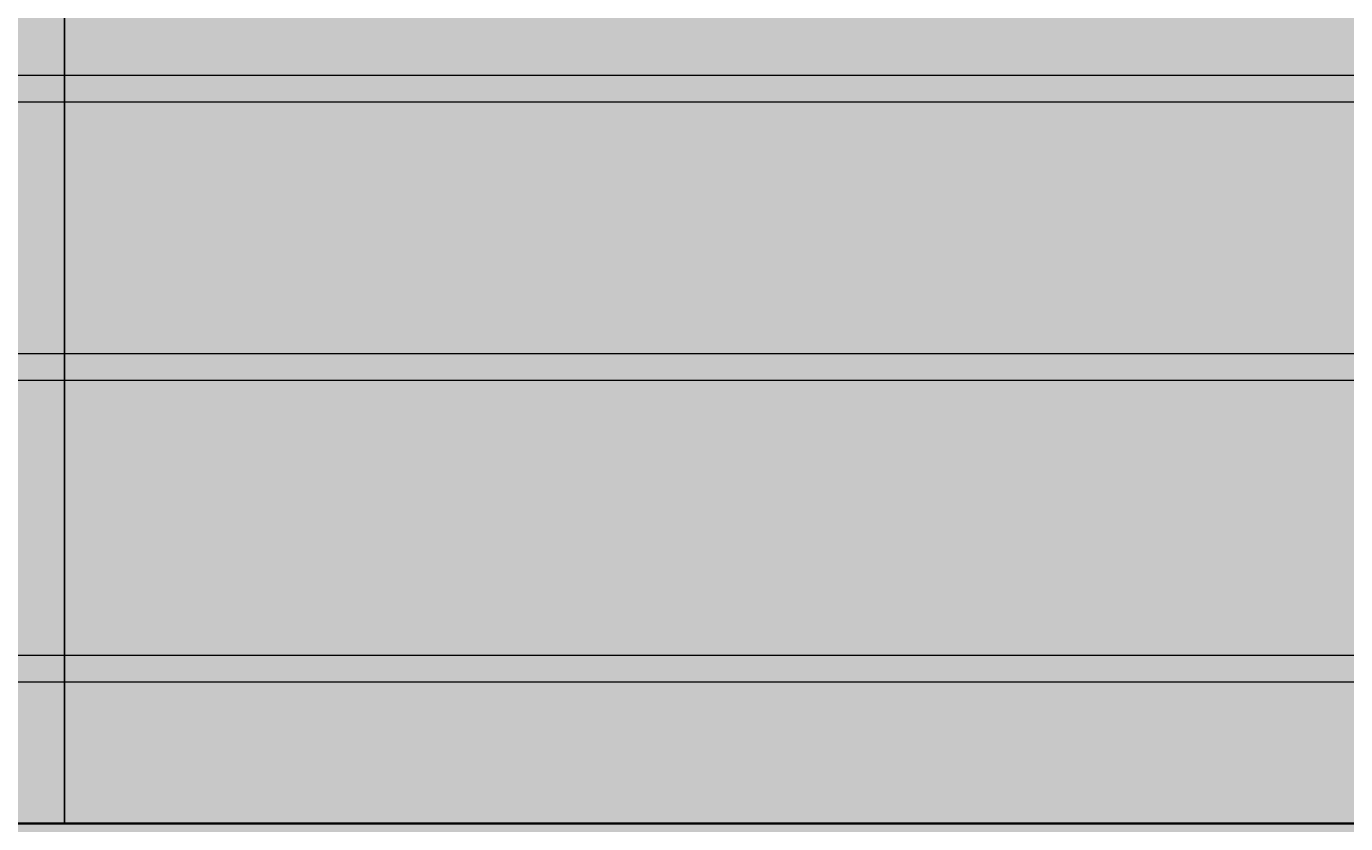
# Model space of a CAD drawing. Units: feet. Extents: x 2695 to 2912, y 795 to 1139.
# Tile 57 of 83: x 2843 to 2877, y 937 to 958. Entities that reach past the tile are written whole.
import ezdxf

# ---------------------------------------------------------------- set-up
doc = ezdxf.new("R2010")
doc.units = ezdxf.units.FT
for name, color, linetype, lineweight in [('A-ANNO-DIMS', 2, 'Continuous', 18), ('A-ELEV', 7, 'Continuous', 35), ('A-ELEV-PATT', 252, 'Continuous', 13), ('A-ELEV-RAIL', 8, 'Continuous', 18), ('A-GLAZ', 4, 'Continuous', 25)]:
    doc.layers.add(name, color=color, linetype=linetype, lineweight=lineweight)
doc.styles.get("Standard").update_dxf_attribs({"font": 'arial.ttf'})
doc.dimstyles.get("Standard").update_dxf_attribs({"dimtxt": 0.18, "dimasz": 0.18, "dimexe": 0.18, "dimexo": 0.0625, "dimgap": 0.09, "dimtad": 0, "dimtih": 1, "dimtoh": 1, "dimdec": 1, "dimzin": 0, "dimdsep": 46, "dimlunit": 3, "dimtxsty": 'Standard', "dimcen": 0.09, "dimadec": 0, "dimazin": 0, "dimtfac": 1, "dimtdec": 1, "dimtofl": 0, "dimtmove": 0, "dimatfit": 3, "dimfxl": 1, "dimtolj": 1, "dimtzin": 0, "dimarcsym": 0})

# ---------------------------------------------------------------- blocks, each defined once
blk = doc.blocks.new('*D17')
at = {"layer": 'A-ANNO-DIMS', "color": 0, "lineweight": -2, "transparency": 16777216}
for p, q in [((2843.637, 1020.824), (2911.424, 1020.824)), ((2911.244, 1020.644), (2911.244, 979.059)), ((2911.244, 937.111), (2911.244, 978.695)), ((2890.699, 936.931), (2911.424, 936.931))]:
    blk.add_line(p, q, dxfattribs=at)
at = {"layer": 'A-ANNO-DIMS', "color": 0, "transparency": 16777216}
for points in [[(2911.214, 1020.644), (2911.274, 1020.644), (2911.244, 1020.824)], [(2911.214, 937.111), (2911.274, 937.111), (2911.244, 936.931)]]:
    blk.add_solid(points, dxfattribs=at)
at = {"layer": 'Defpoints', "color": 0, "transparency": 16777216}
for p in [(2843.575, 1020.824), (2911.244, 1020.824), (2890.636, 936.931)]:
    blk.add_point(p, dxfattribs=at)
at = {"layer": 'A-ANNO-DIMS', "color": 0, "transparency": 16777216, "insert": (2911.244, 978.877), "char_height": 0.18, "attachment_point": 5}
blk.add_mtext('\\A1;83.9', dxfattribs=at)

msp = doc.modelspace()

# ---------------------------------------------------------------- hatches: boundary and pattern name
at = {"layer": 'A-ELEV-PATT'}
h = msp.add_hatch(color=256, dxfattribs=at)
h.set_gradient(color1=(255, 255, 255), tint=1)
h.paths.add_polyline_path([(2770.6361, 1122.9306), (2710.6361, 1122.9306), (2710.6361, 1118.4096), (2770.6361, 1118.4096)])
h.paths.add_polyline_path([(2890.6361, 1107.8588), (2770.6361, 1107.8588), (2770.6361, 1103.3378), (2890.6361, 1103.3378)])
h.paths.add_polyline_path([(2890.6361, 1062.9306), (2710.6361, 1062.9306), (2710.6361, 1056.9306), (2710.6361, 936.9306), (2710.6361, 924.3105), (2716.5358, 924.3105), (2890.6361, 924.3105), (2890.6361, 936.9306), (2715.8852, 936.9306), (2715.8852, 1050.3105), (2890.6361, 1050.3105)])
h.paths.add_polyline_path([(2716.5358, 924.3105), (2710.6361, 924.3105), (2710.6361, 810.9306), (2716.5358, 810.9306)])
h = msp.add_hatch(color=256, dxfattribs=at)
h.set_gradient(color1=(147, 149, 152), color2=(147, 149, 152), tint=1)
h.paths.add_polyline_path([(2770.6361, 1118.4096), (2710.6361, 1118.4096), (2710.6361, 1062.9306), (2770.6361, 1062.9306)])
h.paths.add_polyline_path([(2890.6361, 1103.3378), (2770.6361, 1103.3378), (2770.6361, 1062.9306), (2890.6361, 1062.9306)])
h.paths.add_polyline_path([(2730.7081, 1048.1052), (2755.1125, 1048.1052), (2755.1125, 936.9306), (2770.6361, 936.9306), (2770.6361, 1050.3105), (2715.8852, 1050.3105), (2715.8852, 936.9306), (2730.7081, 936.9306)])
h.paths.add_polyline_path([(2890.6361, 1050.3105), (2770.6361, 1050.3105), (2770.6361, 971.9673), (2778.0341, 971.9673), (2778.0341, 1020.8235), (2843.575, 1020.8235), (2843.575, 971.9673), (2890.6361, 971.9673)])
h.paths.add_polyline_path([(2888.1882, 970.7156), (2843.575, 970.7156), (2843.575, 964.8267), (2888.1882, 964.8267)])
h.paths.add_polyline_path([(2888.1882, 964.1328), (2843.575, 964.1328), (2843.575, 956.614), (2888.1882, 956.614)])
h.paths.add_polyline_path([(2888.1882, 955.9202), (2843.575, 955.9202), (2843.575, 949.2892), (2888.1882, 949.2892)])
h.paths.add_polyline_path([(2888.1882, 948.5954), (2843.575, 948.5954), (2843.575, 941.3507), (2888.1882, 941.3507)])
h.paths.add_polyline_path([(2888.1882, 940.6569), (2843.575, 940.6569), (2843.575, 936.9306), (2888.1882, 936.9306)])
h.paths.add_polyline_path([(2890.6361, 970.7156), (2888.9368, 970.7156), (2888.9368, 964.8267), (2890.6361, 964.8267)])
h.paths.add_polyline_path([(2890.6361, 964.1328), (2888.9368, 964.1328), (2888.9368, 956.614), (2890.6361, 956.614)])
h.paths.add_polyline_path([(2890.6361, 955.9202), (2888.9368, 955.9202), (2888.9368, 949.2892), (2890.6361, 949.2892)])
h.paths.add_polyline_path([(2890.6361, 940.6569), (2888.9368, 940.6569), (2888.9368, 936.9306), (2890.6361, 936.9306)])
h.paths.add_polyline_path([(2890.6361, 948.5954), (2888.9368, 948.5954), (2888.9368, 941.3507), (2890.6361, 941.3507)])
h.paths.add_polyline_path([(2772.5216, 970.7156), (2770.6361, 970.7156), (2770.6361, 964.8267), (2772.5216, 964.8267)])
h.paths.add_polyline_path([(2772.5216, 964.1328), (2770.6361, 964.1328), (2770.6361, 956.614), (2772.5216, 956.614)])
h.paths.add_polyline_path([(2772.5216, 955.9202), (2770.6361, 955.9202), (2770.6361, 949.2892), (2772.5216, 949.2892)])
h.paths.add_polyline_path([(2772.5216, 948.5954), (2770.6361, 948.5954), (2770.6361, 941.3507), (2772.5216, 941.3507)])
h.paths.add_polyline_path([(2772.5216, 940.6569), (2770.6361, 940.6569), (2770.6361, 936.9306), (2772.5216, 936.9306)])
h.paths.add_polyline_path([(2778.0341, 940.6569), (2773.2702, 940.6569), (2773.2702, 936.9306), (2778.0341, 936.9306)])
h.paths.add_polyline_path([(2778.0341, 970.7156), (2773.2702, 970.7156), (2773.2702, 964.8267), (2778.0341, 964.8267)])
h.paths.add_polyline_path([(2778.0341, 964.1328), (2773.2702, 964.1328), (2773.2702, 956.614), (2778.0341, 956.614)])
h.paths.add_polyline_path([(2778.0341, 955.9202), (2773.2702, 955.9202), (2773.2702, 949.2892), (2778.0341, 949.2892)])
h.paths.add_polyline_path([(2778.0341, 948.5954), (2773.2702, 948.5954), (2773.2702, 941.3507), (2778.0341, 941.3507)])
h.paths.add_polyline_path([(2810.0407, 940.6569), (2780.0341, 940.6569), (2780.0341, 936.9306), (2810.0407, 936.9306)])
h.paths.add_polyline_path([(2890.6361, 924.3105), (2770.6361, 924.3105), (2770.6361, 810.9306), (2773.5029, 810.9306), (2773.5029, 905.5143), (2805.9398, 905.5143), (2838.3767, 905.5143), (2838.3767, 810.9306), (2890.6361, 810.9306)])
h = msp.add_hatch(color=256, dxfattribs=at)
h.set_gradient(color2=(0, 0, 0), tint=1)
h.paths.add_polyline_path([(2772.5216, 971.9673), (2770.6361, 971.9673), (2770.6361, 970.7156), (2772.5216, 970.7156)])
h.paths.add_polyline_path([(2773.2702, 971.9673), (2772.5216, 971.9673), (2772.5216, 970.7156), (2773.2702, 970.7156)])
h.paths.add_polyline_path([(2778.0341, 971.9673), (2773.2702, 971.9673), (2773.2702, 970.7156), (2778.0341, 970.7156)])
h.paths.add_polyline_path([(2780.0341, 971.9673), (2778.0341, 971.9673), (2778.0341, 970.7156), (2780.0341, 970.7156)])
h.paths.add_polyline_path([(2841.575, 971.9673), (2780.0341, 971.9673), (2780.0341, 970.7156), (2841.575, 970.7156)])
h.paths.add_polyline_path([(2843.575, 971.9673), (2841.575, 971.9673), (2841.575, 970.7156), (2843.575, 970.7156)])
h.paths.add_polyline_path([(2888.1882, 971.9673), (2843.575, 971.9673), (2843.575, 970.7156), (2888.1882, 970.7156)])
h.paths.add_polyline_path([(2888.9368, 971.9673), (2888.1882, 971.9673), (2888.1882, 970.7156), (2888.9368, 970.7156)], flags=17)
h.paths.add_polyline_path([(2890.6361, 971.9673), (2888.9368, 971.9673), (2888.9368, 970.7156), (2890.6361, 970.7156)])
h.paths.add_polyline_path([(2888.9368, 971.9673), (2888.1882, 971.9673), (2888.1882, 964.8267), (2888.9368, 964.8267)])
h.paths.add_polyline_path([(2888.9368, 964.8267), (2888.1882, 964.8267), (2888.1882, 964.1328), (2888.9368, 964.1328)])
h.paths.add_polyline_path([(2890.6361, 964.8267), (2888.9368, 964.8267), (2888.9368, 964.1328), (2890.6361, 964.1328)])
h.paths.add_polyline_path([(2888.1882, 964.8267), (2770.6361, 964.8267), (2770.6361, 964.1328), (2888.1882, 964.1328)])
h.paths.add_polyline_path([(2888.9368, 964.1328), (2888.1882, 964.1328), (2888.1882, 936.9306), (2888.9368, 936.9306)])
h.paths.add_polyline_path([(2890.6361, 956.614), (2888.9368, 956.614), (2888.9368, 955.9202), (2890.6361, 955.9202)])
h.paths.add_polyline_path([(2888.1882, 956.614), (2770.6361, 956.614), (2770.6361, 955.9202), (2888.1882, 955.9202)])
h.paths.add_polyline_path([(2890.6361, 949.2892), (2888.9368, 949.2892), (2888.9368, 948.5954), (2890.6361, 948.5954)])
h.paths.add_polyline_path([(2888.1882, 949.2892), (2770.6361, 949.2892), (2770.6361, 948.5954), (2888.1882, 948.5954)])
h.paths.add_polyline_path([(2890.6361, 941.3507), (2888.9368, 941.3507), (2888.9368, 940.6569), (2890.6361, 940.6569)])
h.paths.add_polyline_path([(2888.1882, 941.3507), (2770.6361, 941.3507), (2770.6361, 940.6569), (2888.1882, 940.6569)])
h.paths.add_polyline_path([(2773.2702, 970.7156), (2772.5216, 970.7156), (2772.5216, 964.8267), (2773.2702, 964.8267)])
h.paths.add_polyline_path([(2773.2702, 964.1328), (2772.5216, 964.1328), (2772.5216, 956.614), (2773.2702, 956.614)])
h.paths.add_polyline_path([(2773.2702, 955.9202), (2772.5216, 955.9202), (2772.5216, 936.9306), (2773.2702, 936.9306)])
h.paths.add_polyline_path([(2810.7893, 970.7156), (2810.0407, 970.7156), (2810.0407, 964.8267), (2810.7893, 964.8267)], flags=17)
h.paths.add_polyline_path([(2810.7893, 964.1328), (2810.0407, 964.1328), (2810.0407, 956.614), (2810.7893, 956.614)], flags=17)
h.paths.add_polyline_path([(2810.7893, 955.9202), (2810.0407, 955.9202), (2810.0407, 949.2892), (2810.7893, 949.2892)], flags=17)
h.paths.add_polyline_path([(2810.7893, 971.9673), (2810.0407, 971.9673), (2810.0407, 941.3507), (2810.7893, 941.3507)])
h.paths.add_polyline_path([(2810.7893, 940.6569), (2810.0407, 940.6569), (2810.0407, 936.9306), (2810.7893, 936.9306)])
h.paths.add_polyline_path([(2780.0341, 1018.8235), (2841.575, 1018.8235), (2841.575, 971.9673), (2843.575, 971.9673), (2843.575, 1020.8235), (2778.0341, 1020.8235), (2778.0341, 971.9673), (2780.0341, 971.9673)])
h.paths.add_polyline_path([(2780.0341, 970.7156), (2778.0341, 970.7156), (2778.0341, 964.8267), (2780.0341, 964.8267)])
h.paths.add_polyline_path([(2780.0341, 964.1328), (2778.0341, 964.1328), (2778.0341, 956.614), (2780.0341, 956.614)])
h.paths.add_polyline_path([(2780.0341, 955.9202), (2778.0341, 955.9202), (2778.0341, 949.2892), (2780.0341, 949.2892)])
h.paths.add_polyline_path([(2780.0341, 948.5954), (2778.0341, 948.5954), (2778.0341, 941.3507), (2780.0341, 941.3507)])
h.paths.add_polyline_path([(2780.0341, 940.6569), (2778.0341, 940.6569), (2778.0341, 936.9306), (2780.0341, 936.9306)])
h.paths.add_polyline_path([(2843.575, 940.6569), (2841.575, 940.6569), (2841.575, 936.9306), (2843.575, 936.9306)])
h.paths.add_polyline_path([(2843.575, 948.5954), (2841.575, 948.5954), (2841.575, 941.3507), (2843.575, 941.3507)])
h.paths.add_polyline_path([(2843.575, 970.7156), (2841.575, 970.7156), (2841.575, 964.8267), (2843.575, 964.8267)])
h.paths.add_polyline_path([(2843.575, 964.1328), (2841.575, 964.1328), (2841.575, 956.614), (2843.575, 956.614)])
h.paths.add_polyline_path([(2843.575, 955.9202), (2841.575, 955.9202), (2841.575, 949.2892), (2843.575, 949.2892)])
h.paths.add_polyline_path([(2805.0538, 874.1057), (2803.9681, 874.1057), (2803.9681, 846.2857), (2805.0538, 846.2857)])
h.paths.add_polyline_path([(2758.1515, 902.577), (2724.1893, 902.577), (2724.1893, 874.8571), (2758.1515, 874.8571)])
h.paths.add_polyline_path([(2726.1893, 900.577), (2756.1515, 900.577), (2756.1515, 876.8571), (2726.1893, 876.8571)], flags=16)
h.paths.add_polyline_path([(2740.7302, 900.577), (2741.6105, 900.577), (2741.6105, 876.8571), (2740.7302, 876.8571)], flags=0)

# ---------------------------------------------------------------- linework, layer by layer
at = {"layer": 'A-ELEV'}
msp.add_line((2715.8852, 936.9306), (2890.6361, 936.9306), dxfattribs=at)
msp.add_line((2715.8852, 936.9306), (2890.6361, 936.9306), dxfattribs=at)
at = {"layer": 'A-ELEV-RAIL'}
for points in [[(2770.6361, 955.9202), (2890.6361, 955.9202), (2890.6361, 956.614), (2770.6361, 956.614)], [(2770.6361, 948.5954), (2890.6361, 948.5954), (2890.6361, 949.2892), (2770.6361, 949.2892)], [(2770.6361, 940.6569), (2890.6361, 940.6569), (2890.6361, 941.3507), (2770.6361, 941.3507)]]:
    msp.add_lwpolyline(points, close=True, dxfattribs=at)
at = {"layer": 'A-GLAZ'}
msp.add_lwpolyline([(2778.0341, 936.9306), (2778.0341, 1020.8235), (2843.575, 1020.8235), (2843.575, 936.9306)], dxfattribs=at)

# ---------------------------------------------------------------- dimensions: what is measured, and where the dimension line sits
at = {"layer": 'A-ANNO-DIMS'}
dim = msp.add_linear_dim(base=(2911.2444, 1020.8235), p1=(2890.6361, 936.9306), p2=(2843.575, 1020.8235), angle=90, dimstyle='Standard', override={"dimdec": 1, "dimlfac": 1, "dimrnd": 0, "dimzin": 0, "dimdsep": 46, "dimlunit": 2}, dxfattribs=at)
dim.commit()
dim.dimension.update_dxf_attribs({"geometry": '*D17', "text_midpoint": (2911.2444, 978.877)})

doc.saveas('drawing.dxf')
